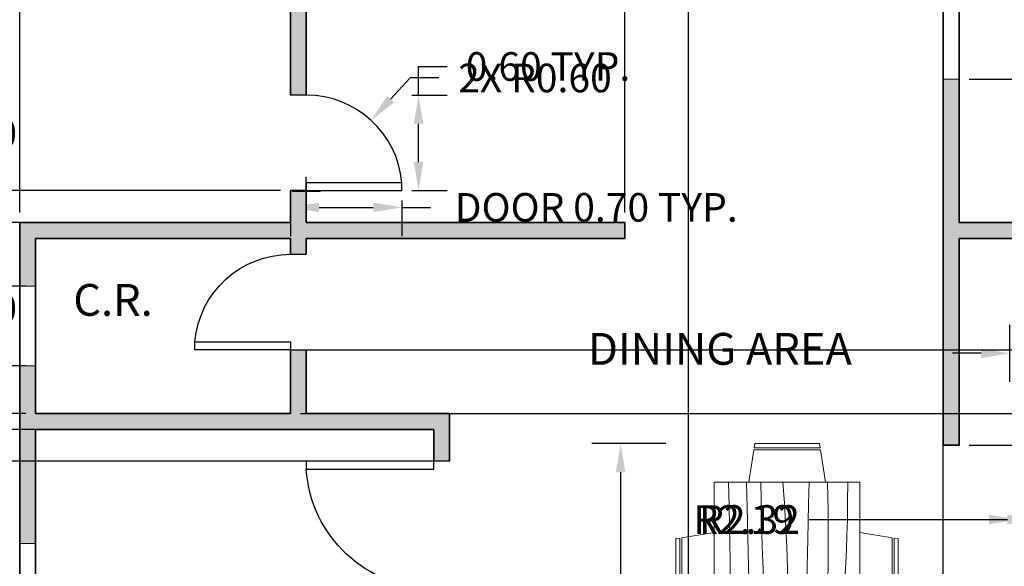
# Model space of a CAD drawing. Units: metres. Extents: x -1.9 to 13.1, y 0.9 to 14.8.
# Tile 5 of 7: x 1.2 to 7.4, y 8.4 to 11.9. Entities that reach past the tile are written whole.
import ezdxf

# ---------------------------------------------------------------- set-up
doc = ezdxf.new("R2010")
doc.units = ezdxf.units.M
doc.header["$MEASUREMENT"] = 0
for name, color, linetype, lineweight in [('A-ANNO-DIMS', 2, 'Continuous', 13), ('A-AREA-IDEN', 7, 'Continuous', 25), ('A-DOOR', 3, 'Continuous', 25), ('A-FURN', 8, 'Continuous', 18), ('A-GLAZ', 4, 'Continuous', 18), ('A-WALL', 7, 'Continuous', 35), ('A-WALL-PATT', 252, 'Continuous', 13)]:
    doc.layers.add(name, color=color, linetype=linetype, lineweight=lineweight)
doc.styles.get("Standard").update_dxf_attribs({"font": 'arial.ttf'})
doc.dimstyles.get("Standard").update_dxf_attribs({"dimtxt": 0.18, "dimasz": 0.18, "dimexe": 0.18, "dimexo": 0.0625, "dimgap": 0.09, "dimtad": 0, "dimtih": 1, "dimtoh": 1, "dimzin": 0, "dimdsep": 46, "dimlunit": 3, "dimtxsty": 'Standard', "dimcen": 0.09, "dimadec": 0, "dimazin": 0, "dimtfac": 1, "dimtofl": 0, "dimtmove": 0, "dimatfit": 3, "dimfxl": 1, "dimtolj": 1, "dimtzin": 0, "dimarcsym": 0})

# ---------------------------------------------------------------- blocks, each defined once
blk = doc.blocks.new('Dining Set - 36 x 72 in.')
for p, q in [((-22, 27.5), (-22.1562, 26.50042)), ((-22, 27.5), (-6, 27.5)), ((-5.8437, 26.49966), (-6, 27.5)), ((6, 27.5), (5.8438, 26.50042)), ((6, 27.5), (22, 27.5)), ((22.1563, 26.49966), (22, 27.5)), ((-22.2343, 26.00059), (-23.4847, 17.99762)), ((-22.2304, 26), (-5.7608, 26)), ((-5.8416, 26.5), (-22.1534, 26.5)), ((-4.5152, 17.99762), (-5.7655, 25.99926)), ((5.7657, 26.00059), (4.5153, 17.99762)), ((5.7696, 26), (22.2392, 26)), ((22.1584, 26.5), (5.8466, 26.5)), ((23.4848, 17.99762), (22.2345, 25.99926)), ((36, 18), (-36, 18)), ((-36, 18), (-36, -18)), ((36, -18), (36, 18)), ((-45.5, 8), (-44.5004, 8.15617)), ((-45.5, 8), (-45.5, -8)), ((-44.5, -8.15843), (-44.5, 8.15338)), ((-44.0006, 8.23428), (-35.9976, 9.48474)), ((-44, 8.23041), (-44, -8.23915)), ((44.0006, 8.23428), (35.9976, 9.48474)), ((44, 8.23041), (44, -8.23915)), ((44.5, -8.15843), (44.5, 8.15338)), ((45.5, 8), (44.5005, 8.15617)), ((45.5, 8), (45.5, -8)), ((-44.4997, -8.15631), (-45.5, -8)), ((-35.9976, -9.48476), (-43.9993, -8.2345)), ((35.9976, -9.48476), (43.9993, -8.2345)), ((44.4997, -8.15631), (45.5, -8)), ((-36, -18), (36, -18)), ((-22.2343, -26.0006), (-23.4847, -17.99762)), ((-4.5152, -17.99762), (-5.7655, -25.99928)), ((5.7657, -26.0006), (4.5153, -17.99762)), ((23.4848, -17.99762), (22.2345, -25.99928)), ((-22.2304, -26), (-5.7608, -26)), ((-22, -27.5), (-22.1562, -26.50044)), ((-5.8416, -26.5), (-22.1534, -26.5)), ((-5.8437, -26.49967), (-6, -27.5)), ((5.7696, -26), (22.2392, -26)), ((6, -27.5), (5.8438, -26.50044)), ((22.1584, -26.5), (5.8466, -26.5)), ((22.1563, -26.49967), (22, -27.5)), ((-22, -27.5), (-6, -27.5)), ((6, -27.5), (22, -27.5))]:
    blk.add_line(p, q)
for points in [[(-36, 15), (-31.1772, 14.97754), (-26.8079, 14.91406), (-22.8538, 14.81543), (-19.276, 14.6875), (-16.0362, 14.53613), (-13.0957, 14.36718), (-10.4159, 14.18652), (-7.9583, 14), (-5.6904, 13.81315), (-3.6035, 13.63021), (-1.6954, 13.45508), (0.0365, 13.29166), (1.5945, 13.14388), (2.9811, 13.01562), (4.1988, 12.9108), (5.25, 12.83333), (6.1393, 12.78613), (6.8802, 12.76823), (7.4883, 12.77767), (7.9792, 12.8125), (8.3685, 12.87077), (8.6719, 12.95052), (8.9049, 13.0498), (9.0833, 13.16666), (9.2205, 13.29899), (9.3216, 13.44401), (9.3895, 13.59879), (9.4271, 13.76041), (9.4373, 13.92594), (9.4232, 14.09245), (9.3875, 14.257), (9.3333, 14.41666), (9.2638, 14.56917), (9.1836, 14.71484), (9.0975, 14.85465), (9.0104, 14.98958), (8.9272, 15.1206), (8.8529, 15.2487), (8.7922, 15.37483), (8.75, 15.5), (8.7305, 15.62467), (8.7344, 15.74739), (8.7617, 15.86621), (8.8125, 15.97916), (8.8867, 16.08431), (8.9844, 16.17968), (9.1055, 16.26334), (9.25, 16.33333), (9.4189, 16.38802), (9.6172, 16.42708), (9.8506, 16.45052), (10.125, 16.45833), (10.4463, 16.45052), (10.8203, 16.42708), (11.2529, 16.38802), (11.75, 16.33333), (12.3184, 16.26318), (12.9694, 16.17838), (13.7151, 16.07991), (14.5677, 15.96875), (15.5395, 15.84586), (16.6426, 15.71224), (17.8893, 15.56884), (19.2917, 15.41666), (20.859, 15.25667), (22.5879, 15.08984), (24.4721, 14.91715), (26.5052, 14.73958), (28.6809, 14.5581), (30.9929, 14.3737), (33.4347, 14.18733), (36, 14)], [(-36, 10), (-28.9766, 10.14274), (-23.1725, 10.20442), (-18.4241, 10.19775), (-14.5677, 10.13541), (-11.4399, 10.03011), (-8.877, 9.89453), (-6.7154, 9.74137), (-4.7917, 9.58333), (-2.9698, 9.43082), (-1.2246, 9.28515), (0.4415, 9.14534), (2.026, 9.01041), (3.5266, 8.87939), (4.9408, 8.7513), (6.266, 8.62516), (7.5, 8.5), (8.6411, 8.37549), (9.6914, 8.2539), (10.6538, 8.13818), (11.5312, 8.03125), (12.3267, 7.93603), (13.043, 7.85547), (13.6831, 7.79248), (14.25, 7.75), (14.7471, 7.7303), (15.1797, 7.73307), (15.5537, 7.75732), (15.875, 7.80208), (16.1494, 7.86637), (16.3828, 7.94922), (16.5811, 8.04964), (16.75, 8.16666), (16.8944, 8.29915), (17.0143, 8.44531), (17.1089, 8.60319), (17.1771, 8.77083), (17.218, 8.94629), (17.2305, 9.1276), (17.2137, 9.31282), (17.1667, 9.5), (17.0895, 9.6875), (16.987, 9.875), (16.8649, 10.0625), (16.7292, 10.25), (16.5856, 10.4375), (16.4401, 10.625), (16.2985, 10.8125), (16.1667, 11), (16.05, 11.18733), (15.9518, 11.3737), (15.8752, 11.5581), (15.8229, 11.73958), (15.798, 11.91715), (15.8034, 12.08984), (15.842, 12.25667), (15.9167, 12.41666), (16.0295, 12.56836), (16.1784, 12.70833), (16.3605, 12.83268), (16.5729, 12.9375), (16.8127, 13.01888), (17.0768, 13.07291), (17.3625, 13.0957), (17.6667, 13.08333), (17.9894, 13.03312), (18.3418, 12.94726), (18.7382, 12.82918), (19.1927, 12.68229), (19.7195, 12.51001), (20.3327, 12.31575), (21.0465, 12.10294), (21.875, 11.875), (22.8357, 11.63354), (23.959, 11.37304), (25.2786, 11.08618), (26.8282, 10.76562), (28.6414, 10.40405), (30.752, 9.99414), (33.1936, 9.52856), (36, 9)], [(-36, 5.5), (-30.7157, 5.3348), (-26.069, 5.20963), (-21.9946, 5.11767), (-18.4271, 5.05208), (-15.3009, 5.00602), (-12.5508, 4.97265), (-10.1112, 4.94515), (-7.9167, 4.91666), (-5.909, 4.88167), (-4.0586, 4.83984), (-2.3429, 4.79215), (-0.7396, 4.73958), (0.7739, 4.6831), (2.22, 4.6237), (3.6213, 4.56233), (5, 4.5), (6.373, 4.43782), (7.7344, 4.3776), (9.0723, 4.32129), (10.375, 4.27083), (11.6309, 4.22819), (12.8281, 4.19531), (13.9551, 4.17415), (15, 4.16666), (15.954, 4.17448), (16.819, 4.19791), (17.6001, 4.23698), (18.3021, 4.29166), (18.9299, 4.36198), (19.4883, 4.44791), (19.9823, 4.54948), (20.4167, 4.66666), (20.7969, 4.79899), (21.1302, 4.94401), (21.4245, 5.09879), (21.6875, 5.26041), (21.9271, 5.42594), (22.1511, 5.59245), (22.3672, 5.757), (22.5834, 5.91666), (22.8065, 6.06868), (23.0404, 6.21093), (23.2879, 6.34147), (23.5521, 6.45833), (23.8358, 6.55957), (24.142, 6.64323), (24.4735, 6.70735), (24.8334, 6.75), (25.2235, 6.76969), (25.642, 6.76692), (26.0858, 6.74267), (26.5521, 6.69791), (27.0379, 6.63362), (27.5404, 6.55078), (28.0565, 6.45036), (28.5834, 6.33333), (29.1242, 6.19987), (29.7071, 6.04687), (30.3661, 5.87044), (31.1354, 5.66666), (32.0493, 5.43164), (33.142, 5.16146), (34.4475, 4.85221), (36, 4.5)], [(-36, -1), (-30.7915, -0.6591), (-26.0195, -0.38216), (-21.6519, -0.16284), (-17.6563, 0.00521), (-14.0005, 0.12833), (-10.6523, 0.21289), (-7.5796, 0.26522), (-4.75, 0.29166), (-2.134, 0.29793), (0.2878, 0.28711), (2.5317, 0.26163), (4.6146, 0.22396), (6.5529, 0.17651), (8.3633, 0.12174), (10.0623, 0.06209), (11.6667, 0), (13.1899, -0.06201), (14.6341, -0.1211), (15.9982, -0.17432), (17.2813, -0.21875), (18.4823, -0.25147), (19.6003, -0.26953), (20.6343, -0.27002), (21.5834, -0.25), (22.4481, -0.20768), (23.2357, -0.14584), (23.9549, -0.06836), (24.6146, 0.02083), (25.2235, 0.11784), (25.7904, 0.21875), (26.3241, 0.31966), (26.8334, 0.41666), (27.3265, 0.50618), (27.8099, 0.58593), (28.2894, 0.65397), (28.7709, 0.70833), (29.2601, 0.74707), (29.763, 0.76823), (30.2855, 0.76985), (30.8334, 0.75), (31.4088, 0.70784), (31.9994, 0.64713), (32.589, 0.57275), (33.1615, 0.48958), (33.7008, 0.4025), (34.1908, 0.3164), (34.6153, 0.23616), (34.9584, 0.16666), (35.2099, 0.11165), (35.3848, 0.07031), (35.504, 0.04069), (35.5886, 0.02083), (35.6594, 0.00879), (35.7377, 0.0026), (35.8442, 0.00032), (36, 0)], [(-36, -6.5), (-27.1843, -6.31267), (-20.084, -6.1263), (-14.469, -5.9419), (-10.1094, -5.76042), (-6.7752, -5.58285), (-4.2363, -5.41016), (-2.2629, -5.24333), (-0.625, -5.08334), (0.8708, -4.93099), (2.2715, -4.78646), (3.5872, -4.64974), (4.8281, -4.52084), (6.0046, -4.39974), (7.127, -4.28646), (8.2053, -4.18099), (9.25, -4.08334), (10.2705, -3.99382), (11.2734, -3.91407), (12.2647, -3.84603), (13.25, -3.79167), (14.2354, -3.75293), (15.2266, -3.73177), (16.2295, -3.73015), (17.25, -3.75), (18.2912, -3.79248), (19.3451, -3.85547), (20.4009, -3.93604), (21.4479, -4.03125), (22.4754, -4.13819), (23.4727, -4.25391), (24.4289, -4.37549), (25.3334, -4.5), (26.1785, -4.62492), (26.9694, -4.74935), (27.7145, -4.87281), (28.4219, -4.99479), (29.1, -5.11483), (29.7572, -5.23242), (30.4016, -5.34709), (31.0417, -5.45834), (31.6837, -5.56437), (32.3262, -5.65821), (32.9658, -5.73153), (33.599, -5.77604), (34.2224, -5.78345), (34.8327, -5.74545), (35.4264, -5.65373), (36, -5.5)], [(-36, -10), (-26.4022, -9.81299), (-18.4675, -9.62891), (-11.9839, -9.45069), (-6.7396, -9.28125), (-2.5226, -9.12354), (0.8789, -8.98047), (3.6769, -8.85498), (6.0833, -8.75), (8.2767, -8.66765), (10.3021, -8.60677), (12.1712, -8.56543), (13.8958, -8.54167), (15.4876, -8.53353), (16.9583, -8.53907), (18.3197, -8.55632), (19.5834, -8.58334), (20.7616, -8.61841), (21.8685, -8.66081), (22.9188, -8.71004), (23.9271, -8.76563), (24.9081, -8.82707), (25.8763, -8.89388), (26.8465, -8.96558), (27.8334, -9.04167), (28.8474, -9.12118), (29.8828, -9.20117), (30.93, -9.27824), (31.9792, -9.34896), (33.0205, -9.40991), (34.0443, -9.45768), (35.0407, -9.48885), (36, -9.5)], [(-36, -14.5), (-30.0881, -14.33513), (-25.0332, -14.21224), (-20.7312, -14.12647), (-17.0781, -14.07292), (-13.97, -14.04671), (-11.3027, -14.04297), (-8.9724, -14.05681), (-6.875, -14.08334), (-4.9224, -14.11833), (-3.0905, -14.16016), (-1.3709, -14.20785), (0.2448, -14.26042), (1.7647, -14.3169), (3.1973, -14.3763), (4.5507, -14.43767), (5.8333, -14.5), (7.0554, -14.5621), (8.235, -14.62175), (9.3922, -14.67652), (10.5469, -14.72396), (11.7192, -14.76164), (12.929, -14.78711), (14.1965, -14.79794), (15.5417, -14.79167), (16.9933, -14.76424), (18.6152, -14.70508), (20.4804, -14.60197), (22.6615, -14.44271), (25.2312, -14.21509), (28.2624, -13.9069), (31.8277, -13.50594), (36, -13)]]:
    blk.add_lwpolyline(points)
blk = doc.blocks.new('*D13')
at = {"layer": 'A-ANNO-DIMS', "color": 0, "lineweight": -2, "transparency": 16777216}
for p, q in [((7.1663, 13.6964), (12.9272, 13.6964)), ((12.7472, 13.5164), (12.7472, 8.3783)), ((12.7472, 2.8764), (12.7472, 8.0145)), ((10.2663, 2.6964), (12.9272, 2.6964))]:
    blk.add_line(p, q, dxfattribs=at)
at = {"layer": 'A-ANNO-DIMS', "color": 0, "transparency": 16777216}
for points in [[(12.7172, 13.5164), (12.7772, 13.5164), (12.7472, 13.6964)], [(12.7172, 2.8764), (12.7772, 2.8764), (12.7472, 2.6964)]]:
    blk.add_solid(points, dxfattribs=at)
at = {"layer": 'Defpoints', "color": 0, "transparency": 16777216}
for p in [(7.1038, 13.6964), (12.7472, 13.6964), (10.2038, 2.6964)]:
    blk.add_point(p, dxfattribs=at)
at = {"layer": 'A-ANNO-DIMS', "color": 0, "transparency": 16777216, "insert": (12.7472, 8.1964), "char_height": 0.18, "attachment_point": 5}
blk.add_mtext('\\A1;11.00"', dxfattribs=at)
blk = doc.blocks.new('*D16')
at = {"layer": 'A-ANNO-DIMS', "color": 0, "lineweight": -2, "transparency": 16777216}
for p, q in [((7.1663, 13.6964), (11.6482, 13.6964)), ((11.4682, 13.5164), (11.4682, 12.3283)), ((11.4682, 10.7764), (11.4682, 11.9644)), ((7.1663, 10.5964), (11.6482, 10.5964))]:
    blk.add_line(p, q, dxfattribs=at)
at = {"layer": 'A-ANNO-DIMS', "color": 0, "transparency": 16777216}
for points in [[(11.4382, 13.5164), (11.4982, 13.5164), (11.4682, 13.6964)], [(11.4382, 10.7764), (11.4982, 10.7764), (11.4682, 10.5964)]]:
    blk.add_solid(points, dxfattribs=at)
at = {"layer": 'Defpoints', "color": 0, "transparency": 16777216}
for p in [(7.1038, 13.6964), (11.4682, 13.6964), (7.1038, 10.5964)]:
    blk.add_point(p, dxfattribs=at)
at = {"layer": 'A-ANNO-DIMS', "color": 0, "transparency": 16777216, "insert": (11.4682, 12.1464), "char_height": 0.18, "attachment_point": 5}
blk.add_mtext('\\A1;3.10"', dxfattribs=at)
blk = doc.blocks.new('*D17')
at = {"layer": 'A-ANNO-DIMS', "color": 0, "lineweight": -2, "transparency": 16777216}
for p, q in [((7.1038, 13.7589), (7.1038, 14.8315)), ((10.2038, 10.6589), (10.2038, 14.8315)), ((7.2838, 14.6515), (8.2857, 14.6515)), ((10.0238, 14.6515), (9.022, 14.6515))]:
    blk.add_line(p, q, dxfattribs=at)
at = {"layer": 'A-ANNO-DIMS', "color": 0, "transparency": 16777216}
for points in [[(7.2838, 14.6815), (7.2838, 14.6215), (7.1038, 14.6515)], [(10.0238, 14.6815), (10.0238, 14.6215), (10.2038, 14.6515)]]:
    blk.add_solid(points, dxfattribs=at)
at = {"layer": 'Defpoints', "color": 0, "transparency": 16777216}
for p in [(7.1038, 14.6515), (7.1038, 13.6964), (10.2038, 10.5964)]:
    blk.add_point(p, dxfattribs=at)
at = {"layer": 'A-ANNO-DIMS', "color": 0, "transparency": 16777216, "insert": (8.6538, 14.6515), "char_height": 0.18, "attachment_point": 5}
blk.add_mtext('\\A1;3.10"', dxfattribs=at)
blk = doc.blocks.new('*D19')
at = {"layer": 'A-ANNO-DIMS', "color": 0, "lineweight": -2, "transparency": 16777216}
for p, q in [((1.2038, 10.6589), (1.2038, 14.8321)), ((2.9038, 13.7589), (2.9038, 14.8321)), ((1.3838, 14.6521), (1.6941, 14.6521)), ((2.7238, 14.6521), (2.4136, 14.6521))]:
    blk.add_line(p, q, dxfattribs=at)
at = {"layer": 'A-ANNO-DIMS', "color": 0, "transparency": 16777216}
for points in [[(1.3838, 14.6821), (1.3838, 14.6221), (1.2038, 14.6521)], [(2.7238, 14.6821), (2.7238, 14.6221), (2.9038, 14.6521)]]:
    blk.add_solid(points, dxfattribs=at)
at = {"layer": 'Defpoints', "color": 0, "transparency": 16777216}
for p in [(1.2038, 14.6521), (2.9038, 13.6964), (1.2038, 10.5964)]:
    blk.add_point(p, dxfattribs=at)
at = {"layer": 'A-ANNO-DIMS', "color": 0, "transparency": 16777216, "insert": (2.0538, 14.6521), "char_height": 0.18, "attachment_point": 5}
blk.add_mtext('\\A1;1.70"', dxfattribs=at)
blk = doc.blocks.new('*D20')
at = {"layer": 'A-ANNO-DIMS', "color": 0, "lineweight": -2, "transparency": 16777216}
for p, q in [((1.1413, 10.5964), (-1.7723, 10.5964)), ((-1.5923, 10.4164), (-1.5923, 6.8283)), ((-1.5923, 2.8764), (-1.5923, 6.4645)), ((1.1413, 2.6964), (-1.7723, 2.6964))]:
    blk.add_line(p, q, dxfattribs=at)
at = {"layer": 'A-ANNO-DIMS', "color": 0, "transparency": 16777216}
for points in [[(-1.6223, 10.4164), (-1.5623, 10.4164), (-1.5923, 10.5964)], [(-1.6223, 2.8764), (-1.5623, 2.8764), (-1.5923, 2.6964)]]:
    blk.add_solid(points, dxfattribs=at)
at = {"layer": 'Defpoints', "color": 0, "transparency": 16777216}
for p in [(1.2038, 10.5964), (-1.5923, 2.6964), (1.2038, 2.6964)]:
    blk.add_point(p, dxfattribs=at)
at = {"layer": 'A-ANNO-DIMS', "color": 0, "transparency": 16777216, "insert": (-1.5923, 6.6464), "char_height": 0.18, "attachment_point": 5}
blk.add_mtext('\\A1;7.90"', dxfattribs=at)
blk = doc.blocks.new('*D21')
at = {"layer": 'A-ANNO-DIMS', "color": 0, "lineweight": -2, "transparency": 16777216}
for p, q in [((1.1413, 10.5964), (-0.3866, 10.5964)), ((-0.2066, 10.4164), (-0.2066, 10.1783)), ((-0.2066, 9.5764), (-0.2066, 9.8145)), ((1.1413, 9.3964), (-0.3866, 9.3964))]:
    blk.add_line(p, q, dxfattribs=at)
at = {"layer": 'A-ANNO-DIMS', "color": 0, "transparency": 16777216}
for points in [[(-0.2366, 10.4164), (-0.1766, 10.4164), (-0.2066, 10.5964)], [(-0.2366, 9.5764), (-0.1766, 9.5764), (-0.2066, 9.3964)]]:
    blk.add_solid(points, dxfattribs=at)
at = {"layer": 'Defpoints', "color": 0, "transparency": 16777216}
for p in [(1.2038, 10.5964), (-0.2066, 9.3964), (1.2038, 9.3964)]:
    blk.add_point(p, dxfattribs=at)
at = {"layer": 'A-ANNO-DIMS', "color": 0, "transparency": 16777216, "insert": (-0.2066, 9.9964), "char_height": 0.18, "attachment_point": 5}
blk.add_mtext('\\A1;1.20"', dxfattribs=at)
blk = doc.blocks.new('*D22')
at = {"layer": 'A-ANNO-DIMS', "color": 0, "lineweight": -2, "transparency": 16777216}
for p, q in [((1.1413, 9.2964), (-0.3896, 9.2964)), ((-0.2096, 9.1164), (-0.2096, 7.7756)), ((-0.2096, 6.0709), (-0.2096, 7.4117)), ((1.1413, 5.8909), (-0.3896, 5.8909))]:
    blk.add_line(p, q, dxfattribs=at)
at = {"layer": 'A-ANNO-DIMS', "color": 0, "transparency": 16777216}
for points in [[(-0.2396, 9.1164), (-0.1796, 9.1164), (-0.2096, 9.2964)], [(-0.2396, 6.0709), (-0.1796, 6.0709), (-0.2096, 5.8909)]]:
    blk.add_solid(points, dxfattribs=at)
at = {"layer": 'Defpoints', "color": 0, "transparency": 16777216}
for p in [(1.2038, 9.2964), (-0.2096, 5.8909), (1.2038, 5.8909)]:
    blk.add_point(p, dxfattribs=at)
at = {"layer": 'A-ANNO-DIMS', "color": 0, "transparency": 16777216, "insert": (-0.2096, 7.5936), "char_height": 0.18, "attachment_point": 5}
blk.add_mtext('\\A1;3.41"', dxfattribs=at)
blk = doc.blocks.new('DOOR-600')
for p, q in [((0.1, 0.6), (0, 0.6)), ((0.1, 0), (0, 0)), ((0.7, 0.05), (0.1, 0.05)), ((0.1, 0.05), (0.1, 0)), ((0.1, 0), (0.7, 0)), ((0.7, 0), (0.7, 0.05))]:
    blk.add_line(p, q)
blk.add_arc((0.1, -0.0023), 0.6023, 4.97911, 90)
blk = doc.blocks.new('DOOR-800')
for p, q in [((0, 0.9), (0, 0.8)), ((0.8, 0.9), (0.8, 0.8)), ((0.75, 0), (0.75, 0.8)), ((0.75, 0.8), (0.8, 0.8)), ((0.8, 0.8), (0.8, 0)), ((0.8, 0), (0.75, 0))]:
    blk.add_line(p, q)
blk.add_arc((0.8017, 0.8), 0.8017, 180, 266.30478)
blk = doc.blocks.new('WIN-1800')
for p, q in [((0, 0.1), (0, 0)), ((0.6, 0.1), (0.6, 0)), ((1.2, 0.1), (1.2, 0)), ((1.8, 0.1), (1.8, 0))]:
    blk.add_line(p, q)
blk = doc.blocks.new('*D32')
at = {"layer": 'A-ANNO-DIMS', "color": 0, "lineweight": -2, "transparency": 16777216}
for p, q in [((2.9038, 10.7339), (2.9038, 10.5114)), ((3.6038, 10.7339), (3.6038, 10.5114)), ((3.0838, 10.6914), (3.4238, 10.6914)), ((3.6038, 10.6914), (3.7838, 10.6914))]:
    blk.add_line(p, q, dxfattribs=at)
at = {"layer": 'A-ANNO-DIMS', "color": 0, "transparency": 16777216}
for points in [[(3.0838, 10.7214), (3.0838, 10.6614), (2.9038, 10.6914)], [(3.4238, 10.7214), (3.4238, 10.6614), (3.6038, 10.6914)]]:
    blk.add_solid(points, dxfattribs=at)
at = {"layer": 'Defpoints', "color": 0, "transparency": 16777216}
for p in [(2.9038, 10.7964), (3.6038, 10.7964), (3.6038, 10.6914)]:
    blk.add_point(p, dxfattribs=at)
at = {"layer": 'A-ANNO-DIMS', "color": 0, "transparency": 16777216, "insert": (4.8244, 10.6914), "char_height": 0.18, "attachment_point": 5}
blk.add_mtext('\\A1;DOOR 0.70 TYP.', dxfattribs=at)
blk = doc.blocks.new('*D33')
at = {"layer": 'A-ANNO-DIMS', "color": 0, "lineweight": -2, "transparency": 16777216}
for p, q in [((3.7088, 11.3964), (3.7088, 11.5764)), ((3.7088, 11.5764), (3.8888, 11.5764)), ((3.6663, 11.3964), (3.8888, 11.3964)), ((3.7088, 10.9764), (3.7088, 11.2164)), ((3.6663, 10.7964), (3.8888, 10.7964))]:
    blk.add_line(p, q, dxfattribs=at)
at = {"layer": 'A-ANNO-DIMS', "color": 0, "transparency": 16777216}
for points in [[(3.6788, 11.2164), (3.7388, 11.2164), (3.7088, 11.3964)], [(3.6788, 10.9764), (3.7388, 10.9764), (3.7088, 10.7964)]]:
    blk.add_solid(points, dxfattribs=at)
at = {"layer": 'Defpoints', "color": 0, "transparency": 16777216}
for p in [(3.6038, 11.3964), (3.7088, 11.3964), (3.6038, 10.7964)]:
    blk.add_point(p, dxfattribs=at)
at = {"layer": 'A-ANNO-DIMS', "color": 0, "transparency": 16777216, "insert": (4.5218, 11.5764), "char_height": 0.18, "attachment_point": 5}
blk.add_mtext('\\A1;0.60 TYP.', dxfattribs=at)
blk = doc.blocks.new('*D43')
at = {"layer": 'A-ANNO-DIMS', "color": 0, "lineweight": -2, "transparency": 16777216}
for p, q in [((7.4214, 9.5958), (7.4214, 9.9544)), ((8.1228, 9.5958), (8.1228, 9.9544)), ((7.2414, 9.7744), (7.0614, 9.7744)), ((8.3028, 9.7744), (8.4828, 9.7744))]:
    blk.add_line(p, q, dxfattribs=at)
at = {"layer": 'A-ANNO-DIMS', "color": 0, "transparency": 16777216}
for points in [[(7.2414, 9.8044), (7.2414, 9.7444), (7.4214, 9.7744)], [(8.3028, 9.8044), (8.3028, 9.7444), (8.1228, 9.7744)]]:
    blk.add_solid(points, dxfattribs=at)
at = {"layer": 'Defpoints', "color": 0, "transparency": 16777216}
for p in [(7.4214, 9.7744), (7.4214, 9.5333), (8.1228, 9.5333)]:
    blk.add_point(p, dxfattribs=at)
at = {"layer": 'A-ANNO-DIMS', "color": 0, "transparency": 16777216, "insert": (7.7721, 9.7744), "char_height": 0.18, "attachment_point": 5}
blk.add_mtext('\\A1;0.70', dxfattribs=at)
blk = doc.blocks.new('*D44')
at = {"layer": 'A-ANNO-DIMS', "color": 0, "lineweight": -2, "transparency": 16777216}
for p, q in [((5.262, 9.2068), (4.7978, 9.2068)), ((4.9778, 9.0268), (4.9778, 8.2342)), ((4.9778, 7.0754), (4.9778, 7.8679)), ((5.262, 6.8954), (4.7978, 6.8954))]:
    blk.add_line(p, q, dxfattribs=at)
at = {"layer": 'A-ANNO-DIMS', "color": 0, "transparency": 16777216}
for points in [[(4.9478, 9.0268), (5.0078, 9.0268), (4.9778, 9.2068)], [(4.9478, 7.0754), (5.0078, 7.0754), (4.9778, 6.8954)]]:
    blk.add_solid(points, dxfattribs=at)
at = {"layer": 'Defpoints', "color": 0, "transparency": 16777216}
for p in [(5.3245, 9.2068), (4.9778, 6.8954), (5.3245, 6.8954)]:
    blk.add_point(p, dxfattribs=at)
at = {"layer": 'A-ANNO-DIMS', "color": 0, "transparency": 16777216, "insert": (4.9778, 8.0511), "char_height": 0.18, "attachment_point": 5}
blk.add_mtext('\\A1;DINING SET 2.31', dxfattribs=at)
blk = doc.blocks.new('*D53')
at = {"layer": 'A-ANNO-DIMS', "color": 0, "lineweight": -2, "transparency": 16777216}
for p, q in [((0.4443, 9.8764), (0.4443, 10.0564)), ((0.4443, 10.0564), (0.6243, 10.0564)), ((1.2413, 9.6964), (0.2643, 9.6964)), ((1.2413, 9.3964), (0.2643, 9.3964)), ((0.4443, 9.2164), (0.4443, 9.0364))]:
    blk.add_line(p, q, dxfattribs=at)
at = {"layer": 'A-ANNO-DIMS', "color": 0, "transparency": 16777216}
for points in [[(0.4143, 9.8764), (0.4743, 9.8764), (0.4443, 9.6964)], [(0.4143, 9.2164), (0.4743, 9.2164), (0.4443, 9.3964)]]:
    blk.add_solid(points, dxfattribs=at)
at = {"layer": 'Defpoints', "color": 0, "transparency": 16777216}
for p in [(0.4443, 9.6964), (1.3038, 9.6964), (1.3038, 9.3964)]:
    blk.add_point(p, dxfattribs=at)
at = {"layer": 'A-ANNO-DIMS', "color": 0, "transparency": 16777216, "insert": (0.9478, 10.0564), "char_height": 0.18, "attachment_point": 5}
blk.add_mtext('\\A1;0.30', dxfattribs=at)
blk = doc.blocks.new('*D54')
at = {"layer": 'A-ANNO-DIMS', "color": 0, "lineweight": -2, "transparency": 16777216}
for p, q in [((0.444347, 10.376378), (0.444347, 10.556378)), ((1.241347, 10.196378), (0.264347, 10.196378)), ((1.241347, 9.696378), (0.264347, 9.696378)), ((0.444347, 9.516378), (0.444347, 9.336378))]:
    blk.add_line(p, q, dxfattribs=at)
at = {"layer": 'A-ANNO-DIMS', "color": 0, "transparency": 16777216}
for points in [[(0.414347, 10.376378), (0.474347, 10.376378), (0.444347, 10.196378)], [(0.414347, 9.516378), (0.474347, 9.516378), (0.444347, 9.696378)]]:
    blk.add_solid(points, dxfattribs=at)
at = {"layer": 'Defpoints', "color": 0, "transparency": 16777216}
for p in [(0.444347, 10.196378), (1.303847, 10.196378), (1.303847, 9.696378)]:
    blk.add_point(p, dxfattribs=at)
at = {"layer": 'A-ANNO-DIMS', "color": 0, "transparency": 16777216, "insert": (0.444347, 9.946378), "char_height": 0.18, "attachment_point": 5}
blk.add_mtext('\\A1;0.50', dxfattribs=at)
blk = doc.blocks.new('*D61')
at = {"layer": 'A-ANNO-DIMS', "color": 0, "lineweight": -2, "transparency": 16777216}
for p, q in [((7.1663, 12.6964), (11.1433, 12.6964)), ((10.9633, 12.5164), (10.9633, 12.2783)), ((10.9633, 11.6764), (10.9633, 11.9145)), ((7.1663, 11.4964), (11.1433, 11.4964))]:
    blk.add_line(p, q, dxfattribs=at)
at = {"layer": 'A-ANNO-DIMS', "color": 0, "transparency": 16777216}
for points in [[(10.9333, 12.5164), (10.9933, 12.5164), (10.9633, 12.6964)], [(10.9333, 11.6764), (10.9933, 11.6764), (10.9633, 11.4964)]]:
    blk.add_solid(points, dxfattribs=at)
at = {"layer": 'Defpoints', "color": 0, "transparency": 16777216}
for p in [(7.1038, 12.6964), (7.1038, 11.4964), (10.9633, 11.4964)]:
    blk.add_point(p, dxfattribs=at)
at = {"layer": 'A-ANNO-DIMS', "color": 0, "transparency": 16777216, "insert": (10.9633, 12.0964), "char_height": 0.18, "attachment_point": 5}
blk.add_mtext('\\A1;1.20', dxfattribs=at)
blk = doc.blocks.new('*D62')
at = {"layer": 'A-ANNO-DIMS', "color": 0, "lineweight": -2, "transparency": 16777216}
for p, q in [((0.4443, 10.9764), (0.4443, 11.1564)), ((0.4443, 11.1564), (0.6243, 11.1564)), ((2.8413, 10.7964), (0.2643, 10.7964)), ((2.8413, 10.5964), (0.2643, 10.5964)), ((0.4443, 10.4164), (0.4443, 10.2364))]:
    blk.add_line(p, q, dxfattribs=at)
at = {"layer": 'A-ANNO-DIMS', "color": 0, "transparency": 16777216}
for points in [[(0.4143, 10.9764), (0.4743, 10.9764), (0.4443, 10.7964)], [(0.4143, 10.4164), (0.4743, 10.4164), (0.4443, 10.5964)]]:
    blk.add_solid(points, dxfattribs=at)
at = {"layer": 'Defpoints', "color": 0, "transparency": 16777216}
for p in [(0.4443, 10.7964), (2.9038, 10.7964), (2.9038, 10.5964)]:
    blk.add_point(p, dxfattribs=at)
at = {"layer": 'A-ANNO-DIMS', "color": 0, "transparency": 16777216, "insert": (0.9478, 11.1564), "char_height": 0.18, "attachment_point": 5}
blk.add_mtext('\\A1;0.20', dxfattribs=at)
blk = doc.blocks.new('*D63')
at = {"layer": 'A-ANNO-DIMS', "color": 0, "lineweight": -2, "transparency": 16777216}
for p, q in [((0.4443, 9.4764), (0.4443, 9.6564)), ((3.7413, 9.2964), (0.2643, 9.2964)), ((3.7413, 9.0964), (0.2643, 9.0964)), ((0.4443, 8.9164), (0.4443, 8.7364)), ((0.4443, 8.7364), (0.2643, 8.7364))]:
    blk.add_line(p, q, dxfattribs=at)
at = {"layer": 'A-ANNO-DIMS', "color": 0, "transparency": 16777216}
for points in [[(0.4143, 9.4764), (0.4743, 9.4764), (0.4443, 9.2964)], [(0.4143, 8.9164), (0.4743, 8.9164), (0.4443, 9.0964)]]:
    blk.add_solid(points, dxfattribs=at)
at = {"layer": 'Defpoints', "color": 0, "transparency": 16777216}
for p in [(3.8038, 9.2964), (0.4443, 9.0964), (3.8038, 9.0964)]:
    blk.add_point(p, dxfattribs=at)
at = {"layer": 'A-ANNO-DIMS', "color": 0, "transparency": 16777216, "insert": (-0.0591, 8.7364), "char_height": 0.18, "attachment_point": 5}
blk.add_mtext('\\A1;0.20', dxfattribs=at)
blk = doc.blocks.new('*D65')
at = {"layer": 'A-ANNO-DIMS', "color": 0, "lineweight": -2, "transparency": 16777216}
for p, q in [((10.963347, 9.976378), (10.963347, 10.156378)), ((2.966347, 9.796378), (11.143347, 9.796378)), ((2.966347, 9.396378), (11.143347, 9.396378)), ((10.963347, 9.216378), (10.963347, 9.036378))]:
    blk.add_line(p, q, dxfattribs=at)
at = {"layer": 'A-ANNO-DIMS', "color": 0, "transparency": 16777216}
for points in [[(10.933347, 9.976378), (10.993347, 9.976378), (10.963347, 9.796378)], [(10.933347, 9.216378), (10.993347, 9.216378), (10.963347, 9.396378)]]:
    blk.add_solid(points, dxfattribs=at)
at = {"layer": 'Defpoints', "color": 0, "transparency": 16777216}
for p in [(2.903847, 9.796378), (2.903847, 9.396378), (10.963347, 9.396378)]:
    blk.add_point(p, dxfattribs=at)
at = {"layer": 'A-ANNO-DIMS', "color": 0, "transparency": 16777216, "insert": (10.963347, 9.596378), "char_height": 0.18, "attachment_point": 5}
blk.add_mtext('\\A1;0.40', dxfattribs=at)
blk = doc.blocks.new('*D66')
at = {"layer": 'A-ANNO-DIMS', "color": 0, "lineweight": -2, "transparency": 16777216}
for p, q in [((5.403847, 4.558878), (5.403847, 14.635878)), ((7.003847, 4.558878), (7.003847, 14.635878)), ((5.583847, 14.455878), (5.888847, 14.455878)), ((6.823847, 14.455878), (6.518847, 14.455878))]:
    blk.add_line(p, q, dxfattribs=at)
at = {"layer": 'A-ANNO-DIMS', "color": 0, "transparency": 16777216}
for points in [[(5.583847, 14.485878), (5.583847, 14.425878), (5.403847, 14.455878)], [(6.823847, 14.485878), (6.823847, 14.425878), (7.003847, 14.455878)]]:
    blk.add_solid(points, dxfattribs=at)
at = {"layer": 'Defpoints', "color": 0, "transparency": 16777216}
for p in [(7.003847, 14.455878), (5.403847, 4.496378), (7.003847, 4.496378)]:
    blk.add_point(p, dxfattribs=at)
at = {"layer": 'A-ANNO-DIMS', "color": 0, "transparency": 16777216, "insert": (6.203847, 14.455878), "char_height": 0.18, "attachment_point": 5}
blk.add_mtext('\\A1;1.60', dxfattribs=at)
blk = doc.blocks.new('*D73')
at = {"layer": 'A-ANNO-DIMS', "color": 0, "lineweight": -2, "transparency": 16777216}
for p, q in [((5.0038, 10.6589), (5.0038, 14.6359)), ((7.0038, 9.2589), (7.0038, 14.6359)), ((5.1838, 14.4559), (5.6788, 14.4559)), ((6.8238, 14.4559), (6.3289, 14.4559))]:
    blk.add_line(p, q, dxfattribs=at)
at = {"layer": 'A-ANNO-DIMS', "color": 0, "transparency": 16777216}
for points in [[(5.1838, 14.4859), (5.1838, 14.4259), (5.0038, 14.4559)], [(6.8238, 14.4859), (6.8238, 14.4259), (7.0038, 14.4559)]]:
    blk.add_solid(points, dxfattribs=at)
at = {"layer": 'Defpoints', "color": 0, "transparency": 16777216}
for p in [(7.0038, 14.4559), (5.0038, 10.5964), (7.0038, 9.1964)]:
    blk.add_point(p, dxfattribs=at)
at = {"layer": 'A-ANNO-DIMS', "color": 0, "transparency": 16777216, "insert": (6.0038, 14.4559), "char_height": 0.18, "attachment_point": 5}
blk.add_mtext('\\A1;2.00', dxfattribs=at)
blk = doc.blocks.new('*D74')
at = {"layer": 'A-ANNO-DIMS', "color": 0, "lineweight": -2, "transparency": 16777216}
for p, q in [((7.1663, 10.4964), (11.1433, 10.4964)), ((10.9633, 10.3164), (10.9633, 10.0283)), ((10.9633, 9.3764), (10.9633, 9.6644)), ((7.1663, 9.1964), (11.1433, 9.1964))]:
    blk.add_line(p, q, dxfattribs=at)
at = {"layer": 'A-ANNO-DIMS', "color": 0, "transparency": 16777216}
for points in [[(10.9333, 10.3164), (10.9933, 10.3164), (10.9633, 10.4964)], [(10.9333, 9.3764), (10.9933, 9.3764), (10.9633, 9.1964)]]:
    blk.add_solid(points, dxfattribs=at)
at = {"layer": 'Defpoints', "color": 0, "transparency": 16777216}
for p in [(7.1038, 10.4964), (10.9633, 10.4964), (7.1038, 9.1964)]:
    blk.add_point(p, dxfattribs=at)
at = {"layer": 'A-ANNO-DIMS', "color": 0, "transparency": 16777216, "insert": (10.9633, 9.8464), "char_height": 0.18, "attachment_point": 5}
blk.add_mtext('\\A1;1.30', dxfattribs=at)
blk = doc.blocks.new('*D77')
at = {"layer": 'A-ANNO-DIMS', "color": 0, "lineweight": -2, "transparency": 16777216}
for p, q in [((3.6552, 11.5043), (3.5326, 11.3706)), ((3.8352, 11.5043), (3.6552, 11.5043)), ((3.0038, 10.7041), (3.0038, 10.8841)), ((2.9138, 10.7941), (3.0938, 10.7941))]:
    blk.add_line(p, q, dxfattribs=at)
at = {"layer": 'A-ANNO-DIMS', "color": 0, "transparency": 16777216}
blk.add_solid([(3.5105, 11.3909), (3.5547, 11.3503), (3.411, 11.2379)], dxfattribs=at)
at = {"layer": 'Defpoints', "color": 0, "transparency": 16777216}
for p in [(3.411, 11.2379), (3.0038, 10.7941)]:
    blk.add_point(p, dxfattribs=at)
at = {"layer": 'A-ANNO-DIMS', "color": 0, "transparency": 16777216, "insert": (4.4397, 11.5043), "char_height": 0.18, "attachment_point": 5}
blk.add_mtext('\\A1;2X R0.60', dxfattribs=at)
blk = doc.blocks.new('*D78')
at = {"layer": 'A-ANNO-DIMS', "color": 0, "lineweight": -2, "transparency": 16777216}
for p, q in [((9.9057, 8.6399), (9.9057, 8.8199)), ((6.1961, 8.7301), (7.4072, 8.73)), ((9.8157, 8.7299), (9.9957, 8.7299))]:
    blk.add_line(p, q, dxfattribs=at)
at = {"layer": 'A-ANNO-DIMS', "color": 0, "transparency": 16777216}
blk.add_solid([(7.4072, 8.76), (7.4072, 8.7), (7.5872, 8.73)], dxfattribs=at)
at = {"layer": 'Defpoints', "color": 0, "transparency": 16777216}
for p in [(7.5872, 8.73), (9.9057, 8.7299)]:
    blk.add_point(p, dxfattribs=at)
at = {"layer": 'A-ANNO-DIMS', "color": 0, "transparency": 16777216, "insert": (5.7871, 8.7301), "char_height": 0.18, "attachment_point": 5}
blk.add_mtext('\\A1;R2.32', dxfattribs=at)
blk = doc.blocks.new('*D79')
at = {"layer": 'A-ANNO-DIMS', "color": 0, "lineweight": -2, "transparency": 16777216}
for p, q in [((9.658, 8.6399), (9.658, 8.8199)), ((6.161, 8.7301), (7.2924, 8.73)), ((9.568, 8.7299), (9.748, 8.7299))]:
    blk.add_line(p, q, dxfattribs=at)
at = {"layer": 'A-ANNO-DIMS', "color": 0, "transparency": 16777216}
blk.add_solid([(7.2924, 8.76), (7.2924, 8.7), (7.4724, 8.73)], dxfattribs=at)
at = {"layer": 'Defpoints', "color": 0, "transparency": 16777216}
for p in [(7.4724, 8.73), (9.658, 8.7299)]:
    blk.add_point(p, dxfattribs=at)
at = {"layer": 'A-ANNO-DIMS', "color": 0, "transparency": 16777216, "insert": (5.7509, 8.7301), "char_height": 0.18, "attachment_point": 5}
blk.add_mtext('\\A1;R2.19', dxfattribs=at)

msp = doc.modelspace()

# ---------------------------------------------------------------- linework, layer by layer
at = {"layer": 'A-GLAZ'}
for p, q in [((7.1038, 11.4964), (7.0038, 11.4964)), ((1.3038, 10.1964), (1.2038, 10.1964)), ((1.3038, 9.6964), (1.2038, 9.6964))]:
    msp.add_line(p, q, dxfattribs=at)
at = {"layer": 'A-WALL'}
for p, q in [((2.9038, 11.3964), (2.9038, 13.6964)), ((7.1038, 10.5964), (7.1038, 13.6964)), ((3.0038, 11.3964), (3.0038, 13.5964)), ((7.0038, 9.1964), (7.0038, 13.5964)), ((2.9038, 10.5964), (2.9038, 10.7964)), ((3.0038, 10.5964), (3.0038, 10.7964)), ((2.9038, 10.5964), (1.2038, 10.5964)), ((5.0038, 10.5964), (3.0038, 10.5964)), ((5.0038, 10.4964), (5.0038, 10.5964)), ((10.2038, 10.5964), (7.1038, 10.5964)), ((1.3038, 10.4964), (1.3038, 9.3964)), ((2.9038, 10.4964), (1.3038, 10.4964)), ((2.9038, 10.3964), (2.9038, 10.4964)), ((5.0038, 10.4964), (3.0038, 10.4964)), ((3.0038, 10.3964), (3.0038, 10.4964)), ((10.1038, 10.4964), (7.1038, 10.4964)), ((7.1038, 9.1964), (7.1038, 10.4964)), ((2.9038, 9.3964), (2.9038, 9.7964)), ((3.0038, 9.3964), (3.0038, 9.7964)), ((1.3038, 9.3964), (2.9038, 9.3964)), ((3.0038, 9.3964), (3.9038, 9.3964)), ((3.9038, 9.3964), (3.9038, 9.0964)), ((1.3038, 9.2964), (3.8038, 9.2964)), ((1.3038, 9.2964), (1.3038, 5.8964)), ((3.8038, 9.2964), (3.8038, 9.0964)), ((7.1038, 9.1964), (7.0038, 9.1964))]:
    msp.add_line(p, q, dxfattribs=at)
msp.add_lwpolyline([(1.2038, 10.5964), (1.2038, 2.6964), (10.2038, 2.6964), (10.2038, 10.5964)], dxfattribs=at)
at = {"layer": 'A-WALL-PATT'}
for points in [[(2.9038, 11.3964), (3.0038, 11.3964), (2.9038, 13.6964), (3.0038, 13.5964)], [(7.0038, 11.4964), (7.1038, 11.4964), (7.0038, 9.1964), (7.1038, 9.1964)], [(2.9038, 10.7964), (3.0038, 10.7964), (2.9038, 10.3964), (3.0038, 10.3964)], [(1.2038, 10.1964), (1.3038, 10.1964), (1.2038, 10.5964), (1.3038, 10.4964)], [(1.2038, 10.5964), (1.3038, 10.4964), (2.9038, 10.5964), (2.9038, 10.4964)], [(2.9038, 10.5964), (2.9038, 10.4964), (5.0038, 10.5964), (5.0038, 10.4964)], [(7.1038, 10.5964), (7.1038, 10.4964), (10.2038, 10.5964), (10.1038, 10.4964)], [(2.9038, 9.7964), (3.0038, 9.7964), (2.9038, 9.3964), (3.0038, 9.3964)], [(1.2038, 8.5785), (1.3038, 8.5785), (1.2038, 9.6964), (1.3038, 9.6964)], [(1.3038, 9.3964), (1.3038, 9.2964), (3.9038, 9.3964), (3.8038, 9.2964)], [(3.9038, 9.3964), (3.8038, 9.2964), (3.9038, 9.0964), (3.8038, 9.0964)]]:
    msp.add_solid(points, dxfattribs=at)

# ---------------------------------------------------------------- block references
at = {"layer": 'A-DOOR'}
msp.add_blockref('DOOR-600', (2.9038, 10.7964), dxfattribs=at)
at = {"layer": 'A-DOOR', "extrusion": (0, 0, -1), "zscale": -1}
msp.add_blockref('DOOR-600', (-3.0038, 9.7964), dxfattribs=at)
at = {"layer": 'A-DOOR', "extrusion": (0, 0, -1), "zscale": -1, "rotation": 89.99999999999893}
msp.add_blockref('DOOR-800', (-3.0038, 8.2964), dxfattribs=at)
at = {"layer": 'A-FURN', "xscale": 0.0254, "yscale": 0.0254, "zscale": 0.0254, "rotation": 270}
msp.add_blockref('Dining Set - 36 x 72 in.', (6.023, 8.0511), dxfattribs=at)
at = {"layer": 'A-GLAZ', "rotation": 90.00000000000006}
msp.add_blockref('WIN-1800', (1.3038, 6.7785), dxfattribs=at)

# ---------------------------------------------------------------- texts
at = {"layer": 'A-AREA-IDEN', "char_height": 0.2, "attachment_point": 1}
for s, width, insert in [('\\pxqc;C.R.', 0.575474, (1.5021, 10.2099)), ('\\pxqc;DINING AREA', 1.825358, (4.6893, 9.9024))]:
    msp.add_mtext_dynamic_manual_height_columns(s, width=width, gutter_width=1, heights=[0], dxfattribs=dict(at, insert=insert))

# ---------------------------------------------------------------- dimensions: what is measured, and where the dimension line sits
at = {"layer": 'A-ANNO-DIMS'}
for base, p1, p2, override, picture, middle in [((1.2038, 14.6521), (2.9038, 13.6964), (1.2038, 10.5964), {"dimclrd": 0, "dimclre": 0, "dimclrt": 0}, '*D19', (2.0538, 14.6521)), ((7.1038, 14.6515), (10.2038, 10.5964), (7.1038, 13.6964), {"dimclrd": 0, "dimclre": 0, "dimclrt": 0}, '*D17', (8.6538, 14.6515)), ((7.0038, 14.4559), (5.0038, 10.5964), (7.0038, 9.1964), {"dimdec": 2, "dimlfac": 1, "dimrnd": 0, "dimzin": 0, "dimdsep": 46, "dimlunit": 2}, '*D73', (6.0038, 14.4559)), ((7.0038, 14.4559), (5.4038, 4.4964), (7.0038, 4.4964), {"dimdec": 2, "dimlfac": 1, "dimrnd": 0, "dimzin": 0, "dimdsep": 46, "dimlunit": 2}, '*D66', (6.2038, 14.4559))]:
    dim = msp.add_linear_dim(base=base, p1=p1, p2=p2, dimstyle='Standard', override=override, dxfattribs=at)
    dim.commit()
    dim.dimension.update_dxf_attribs({"geometry": picture, "text_midpoint": middle})
for base, p1, p2, angle, override, picture, middle in [((12.7472, 13.6964), (10.2038, 2.6964), (7.1038, 13.6964), 90, {"dimclrd": 0, "dimclre": 0, "dimclrt": 0}, '*D13', (12.7472, 8.1964)), ((11.4682, 13.6964), (7.1038, 10.5964), (7.1038, 13.6964), 90, {"dimclrd": 0, "dimclre": 0, "dimclrt": 0}, '*D16', (11.4682, 12.1464)), ((10.9633, 11.4964), (7.1038, 12.6964), (7.1038, 11.4964), 90, {"dimdec": 2, "dimlfac": 1, "dimrnd": 0, "dimzin": 0, "dimdsep": 46, "dimlunit": 2}, '*D61', (10.9633, 12.0964)), ((0.4443, 10.7964), (2.9038, 10.5964), (2.9038, 10.7964), 90, {"dimdec": 2, "dimlfac": 1, "dimrnd": 0, "dimzin": 0, "dimdsep": 46, "dimlunit": 2}, '*D62', (0.9478, 11.1564)), ((-1.5923, 2.6964), (1.2038, 10.5964), (1.2038, 2.6964), 90, {"dimclrd": 0, "dimclre": 0, "dimclrt": 0}, '*D20', (-1.5923, 6.6464)), ((-0.2066, 9.3964), (1.2038, 10.5964), (1.2038, 9.3964), 90, {"dimclrd": 0, "dimclre": 0, "dimclrt": 0}, '*D21', (-0.2066, 9.9964)), ((0.4443, 10.1964), (1.3038, 9.6964), (1.3038, 10.1964), 90, {"dimdec": 2, "dimlfac": 1, "dimrnd": 0, "dimzin": 0, "dimdsep": 46, "dimlunit": 2}, '*D54', (0.4443, 9.9464)), ((10.9633, 10.4964), (7.1038, 9.1964), (7.1038, 10.4964), 90, {"dimdec": 2, "dimlfac": 1, "dimrnd": 0, "dimzin": 0, "dimdsep": 46, "dimlunit": 2}, '*D74', (10.9633, 9.8464)), ((0.4443, 9.6964), (1.3038, 9.3964), (1.3038, 9.6964), 90, {"dimdec": 2, "dimlfac": 1, "dimrnd": 0, "dimzin": 0, "dimdsep": 46, "dimlunit": 2}, '*D53', (0.9478, 10.0564)), ((10.9633, 9.3964), (2.9038, 9.7964), (2.9038, 9.3964), 90, {"dimdec": 2, "dimlfac": 1, "dimrnd": 0, "dimzin": 0, "dimdsep": 46, "dimlunit": 2}, '*D65', (10.9633, 9.5964)), ((7.4214, 9.7744), (8.1228, 9.5333), (7.4214, 9.5333), 180, {"dimdec": 2, "dimlfac": 1, "dimrnd": 0, "dimzin": 0, "dimdsep": 46, "dimlunit": 2}, '*D43', (7.7721, 9.7744)), ((0.4443, 9.0964), (3.8038, 9.2964), (3.8038, 9.0964), 90, {"dimdec": 2, "dimlfac": 1, "dimrnd": 0, "dimzin": 0, "dimdsep": 46, "dimlunit": 2}, '*D63', (-0.0591, 8.7364)), ((-0.2096, 5.8909), (1.2038, 9.2964), (1.2038, 5.8909), 90, {"dimclrd": 0, "dimclre": 0, "dimclrt": 0}, '*D22', (-0.2096, 7.5936))]:
    dim = msp.add_linear_dim(base=base, p1=p1, p2=p2, angle=angle, dimstyle='Standard', override=override, dxfattribs=at)
    dim.commit()
    dim.dimension.update_dxf_attribs({"geometry": picture, "text_midpoint": middle})
for base, p1, p2, angle, text, picture, middle in [((3.7088, 11.3964), (3.6038, 10.7964), (3.6038, 11.3964), 90, '<> TYP.', '*D33', (4.5218, 11.5764)), ((4.9778, 6.8954), (5.3245, 9.2068), (5.3245, 6.8954), 270, 'DINING SET <>', '*D44', (4.9778, 8.0511))]:
    dim = msp.add_linear_dim(base=base, p1=p1, p2=p2, angle=angle, text=text, dimstyle='Standard', override={"dimdec": 2, "dimlfac": 1, "dimrnd": 0, "dimzin": 0, "dimdsep": 46, "dimlunit": 2}, dxfattribs=at)
    dim.commit()
    dim.dimension.update_dxf_attribs({"geometry": picture, "text_midpoint": middle})
dim = msp.add_radius_dim(center=(3.0038, 10.7941), mpoint=(3.411, 11.2379), text='2X <>', dimstyle='Standard', override={"dimdec": 2, "dimlfac": 1, "dimrnd": 0, "dimzin": 0, "dimdsep": 46, "dimlunit": 2}, dxfattribs=at)
dim.commit()
dim.dimension.update_dxf_attribs({"geometry": '*D77', "text_midpoint": (4.4397, 11.5043), "dimtype": 164})
dim = msp.add_linear_dim(base=(3.6038, 10.6914), p1=(2.9038, 10.7964), p2=(3.6038, 10.7964), text='DOOR <> TYP.', dimstyle='Standard', override={"dimdec": 2, "dimlfac": 1, "dimrnd": 0, "dimzin": 0, "dimdsep": 46, "dimlunit": 2}, dxfattribs=at)
dim.commit()
dim.dimension.update_dxf_attribs({"geometry": '*D32', "text_midpoint": (4.8244, 10.6914)})
for center, mpoint, picture, middle in [((9.658, 8.7299), (7.4724, 8.73), '*D79', (6.161, 8.7301)), ((9.9057, 8.7299), (7.5872, 8.73), '*D78', (6.1961, 8.7301))]:
    dim = msp.add_radius_dim(center=center, mpoint=mpoint, dimstyle='Standard', override={"dimdec": 2, "dimlfac": 1, "dimrnd": 0, "dimzin": 0, "dimdsep": 46, "dimlunit": 2}, dxfattribs=at)
    dim.commit()
    dim.dimension.update_dxf_attribs({"geometry": picture, "text_midpoint": middle, "dimtype": 164})

doc.saveas('drawing.dxf')
